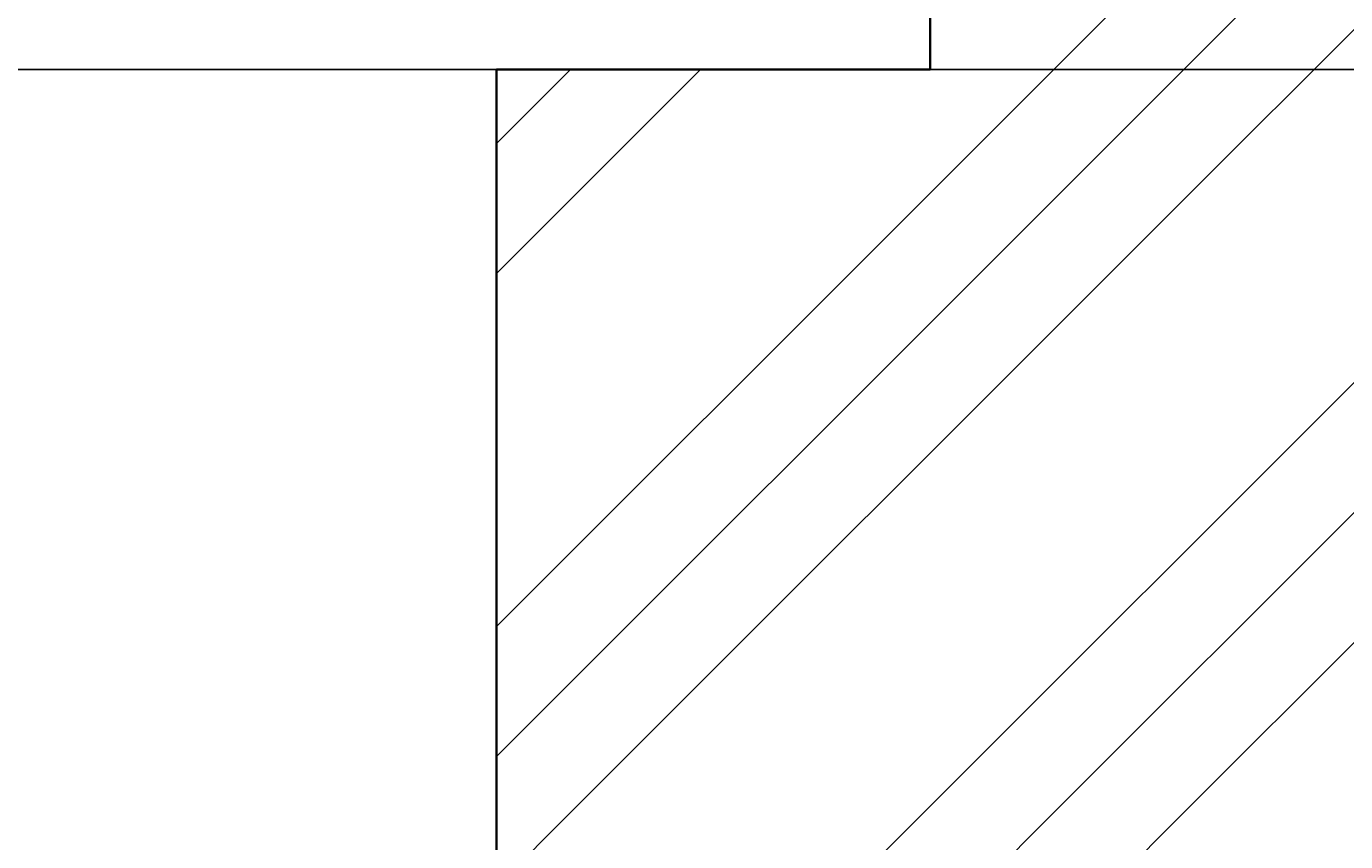
# Model space of a CAD drawing. Units: inches. Extents: x -128 to 854, y -395 to 398.
# Tile 5 of 61: x -77 to -47, y -340 to -321. Entities that reach past the tile are written whole.
import ezdxf

# ---------------------------------------------------------------- set-up
doc = ezdxf.new("R2010")
doc.units = ezdxf.units.IN
doc.header["$MEASUREMENT"] = 0
for name, color, linetype, lineweight in [('A-ANNO-DIMS', 2, 'Continuous', 18), ('A-SECT-PATT', 8, 'Continuous', 13), ('S-FNDN', 2, 'Continuous', 35)]:
    doc.layers.add(name, color=color, linetype=linetype, lineweight=lineweight)
doc.styles.get("Standard").update_dxf_attribs({"font": 'arial.ttf'})
doc.dimstyles.get("Standard").update_dxf_attribs({"dimtxt": 0.18, "dimasz": 0.18, "dimexe": 0.18, "dimexo": 0.0625, "dimgap": 0.09, "dimtad": 0, "dimtih": 1, "dimtoh": 1, "dimdec": 1, "dimzin": 0, "dimdsep": 46, "dimlunit": 4, "dimtxsty": 'Standard', "dimcen": 0.09, "dimclrd": 1, "dimclre": 2, "dimclrt": 6, "dimadec": 0, "dimazin": 0, "dimtfac": 1, "dimtdec": 1, "dimtofl": 0, "dimtmove": 0, "dimatfit": 3, "dimfxl": 1, "dimtfill": 2, "dimtfillclr": 3, "dimtolj": 1, "dimtzin": 0, "dimarcsym": 0})

# ---------------------------------------------------------------- blocks, each defined once
blk = doc.blocks.new('*D121')
at = {"layer": 'A-ANNO-DIMS', "color": 2, "lineweight": -2, "transparency": 16777216}
for p, q in [((-56.223, -298.019), (-128.041, -298.019)), ((-76.223, -358.019), (-128.041, -358.019))]:
    blk.add_line(p, q, dxfattribs=at)
at = {"layer": 'A-ANNO-DIMS', "color": 1, "lineweight": -2, "transparency": 16777216}
for p, q in [((-127.861, -298.199), (-127.861, -327.837)), ((-127.861, -357.839), (-127.861, -328.201))]:
    blk.add_line(p, q, dxfattribs=at)
at = {"layer": 'A-ANNO-DIMS', "color": 1, "transparency": 16777216}
for points in [[(-127.891, -298.199), (-127.831, -298.199), (-127.861, -298.019)], [(-127.891, -357.839), (-127.831, -357.839), (-127.861, -358.019)]]:
    blk.add_solid(points, dxfattribs=at)
at = {"layer": 'Defpoints', "color": 0, "transparency": 16777216}
for p in [(-56.161, -298.019), (-127.861, -358.019), (-76.161, -358.019)]:
    blk.add_point(p, dxfattribs=at)
at = {"layer": 'A-ANNO-DIMS', "color": 6, "transparency": 16777216, "insert": (-127.861, -328.019), "char_height": 0.18, "attachment_point": 5, "bg_fill": 1, "box_fill_scale": 1.25, "bg_fill_color": 3, "bg_fill_transparency": 0}
blk.add_mtext('\\A1;5\'-0"', dxfattribs=at)
blk = doc.blocks.new('*D129')
at = {"layer": 'A-ANNO-DIMS', "color": 2, "lineweight": -2, "transparency": 16777216}
for p, q in [((-27.223, -322.019), (-128.041, -322.019)), ((-27.223, -346.019), (-128.041, -346.019))]:
    blk.add_line(p, q, dxfattribs=at)
at = {"layer": 'A-ANNO-DIMS', "color": 1, "lineweight": -2, "transparency": 16777216}
for p, q in [((-127.861, -322.199), (-127.861, -333.837)), ((-127.861, -345.839), (-127.861, -334.201))]:
    blk.add_line(p, q, dxfattribs=at)
at = {"layer": 'A-ANNO-DIMS', "color": 1, "transparency": 16777216}
for points in [[(-127.891, -322.199), (-127.831, -322.199), (-127.861, -322.019)], [(-127.891, -345.839), (-127.831, -345.839), (-127.861, -346.019)]]:
    blk.add_solid(points, dxfattribs=at)
at = {"layer": 'Defpoints', "color": 0, "transparency": 16777216}
for p in [(-127.861, -322.019), (-27.161, -322.019), (-27.161, -346.019)]:
    blk.add_point(p, dxfattribs=at)
at = {"layer": 'A-ANNO-DIMS', "color": 6, "transparency": 16777216, "insert": (-127.861, -334.019), "char_height": 0.18, "attachment_point": 5, "bg_fill": 1, "box_fill_scale": 1.25, "bg_fill_color": 3, "bg_fill_transparency": 0}
blk.add_mtext('\\A1;2\'-0"', dxfattribs=at)
blk = doc.blocks.new('*D130')
at = {"layer": 'A-ANNO-DIMS', "color": 2, "lineweight": -2, "transparency": 16777216}
for p, q in [((-66.161, -322.082), (-66.161, -381.899)), ((-27.161, -322.082), (-27.161, -381.899))]:
    blk.add_line(p, q, dxfattribs=at)
at = {"layer": 'A-ANNO-DIMS', "color": 1, "lineweight": -2, "transparency": 16777216}
for p, q in [((-65.981, -381.719), (-46.99, -381.719)), ((-27.341, -381.719), (-46.332, -381.719))]:
    blk.add_line(p, q, dxfattribs=at)
at = {"layer": 'A-ANNO-DIMS', "color": 1, "transparency": 16777216}
for points in [[(-65.981, -381.689), (-65.981, -381.749), (-66.161, -381.719)], [(-27.341, -381.689), (-27.341, -381.749), (-27.161, -381.719)]]:
    blk.add_solid(points, dxfattribs=at)
at = {"layer": 'Defpoints', "color": 0, "transparency": 16777216}
for p in [(-66.161, -322.019), (-27.161, -322.019), (-27.161, -381.719)]:
    blk.add_point(p, dxfattribs=at)
at = {"layer": 'A-ANNO-DIMS', "color": 6, "transparency": 16777216, "insert": (-46.661, -381.719), "char_height": 0.18, "attachment_point": 5, "bg_fill": 1, "box_fill_scale": 1.25, "bg_fill_color": 3, "bg_fill_transparency": 0}
blk.add_mtext('\\A1;3\'-3"', dxfattribs=at)

msp = doc.modelspace()

# ---------------------------------------------------------------- hatches: boundary and pattern name
at = {"layer": 'A-SECT-PATT'}
h = msp.add_hatch(dxfattribs=at)
h.set_pattern_fill('GOST_GROUND', color=256)
h.set_pattern_definition([(45, (0, 0), (14.14214, -9e-16), [20]), (45, (3, 0), (14.14214, -9e-16), [20]), (45, (6, 0), (14.14214, -9e-16), [20])])
h.paths.add_polyline_path([(-27.161, -322.019), (-37.161, -322.019), (-37.161, -298.019), (-56.161, -298.019), (-56.161, -322.019), (-66.161, -322.019), (-66.161, -346.019), (-27.161, -346.019)])
h.paths.add_polyline_path([(170.839, -322.019), (160.839, -322.019), (160.839, -298.019), (155.839, -298.019), (141.839, -298.019), (141.839, -322.019), (131.839, -322.019), (131.839, -346.019), (170.839, -346.019)])
h.paths.add_polyline_path([(327.839, -322.019), (317.839, -322.019), (317.839, -298.019), (312.839, -298.019), (298.839, -298.019), (298.839, -322.019), (288.839, -322.019), (288.839, -346.019), (327.839, -346.019)])
h.paths.add_polyline_path([(-37.161, -274.019), (-56.161, -274.019), (-56.161, -298.019), (-37.161, -298.019)])
h.paths.add_polyline_path([(-37.161, -207.019), (-56.161, -207.019), (-56.161, -226.019), (-37.161, -226.019)])
h.paths.add_polyline_path([(160.839, -274.019), (141.839, -274.019), (141.839, -298.019), (155.839, -298.019), (160.839, -298.019)])

# ---------------------------------------------------------------- linework, layer by layer
at = {"layer": 'S-FNDN'}
for p, q in [((-56.161, -298.019), (-56.161, -322.019)), ((-56.161, -322.019), (-66.161, -322.019)), ((-66.161, -322.019), (-66.161, -346.019))]:
    msp.add_line(p, q, dxfattribs=at)

# ---------------------------------------------------------------- dimensions: what is measured, and where the dimension line sits
at = {"layer": 'A-ANNO-DIMS'}
for base, p1, p2, picture, middle in [((-127.861, -358.019), (-56.161, -298.019), (-76.161, -358.019), '*D121', (-127.861, -328.019)), ((-127.861, -322.019), (-27.161, -346.019), (-27.161, -322.019), '*D129', (-127.861, -334.019))]:
    dim = msp.add_linear_dim(base=base, p1=p1, p2=p2, angle=90, dimstyle='Standard', override={"dimdec": 1, "dimlfac": 1, "dimrnd": 0, "dimzin": 1, "dimdsep": 46, "dimlunit": 4, "dimfrac": 2}, dxfattribs=at)
    dim.commit()
    dim.dimension.update_dxf_attribs({"geometry": picture, "text_midpoint": middle})
dim = msp.add_linear_dim(base=(-27.161, -381.719), p1=(-66.161, -322.019), p2=(-27.161, -322.019), dimstyle='Standard', override={"dimdec": 1, "dimlfac": 1, "dimrnd": 0, "dimzin": 1, "dimdsep": 46, "dimlunit": 4, "dimfrac": 2}, dxfattribs=at)
dim.commit()
dim.dimension.update_dxf_attribs({"geometry": '*D130', "text_midpoint": (-46.661, -381.719)})

doc.saveas('drawing.dxf')
